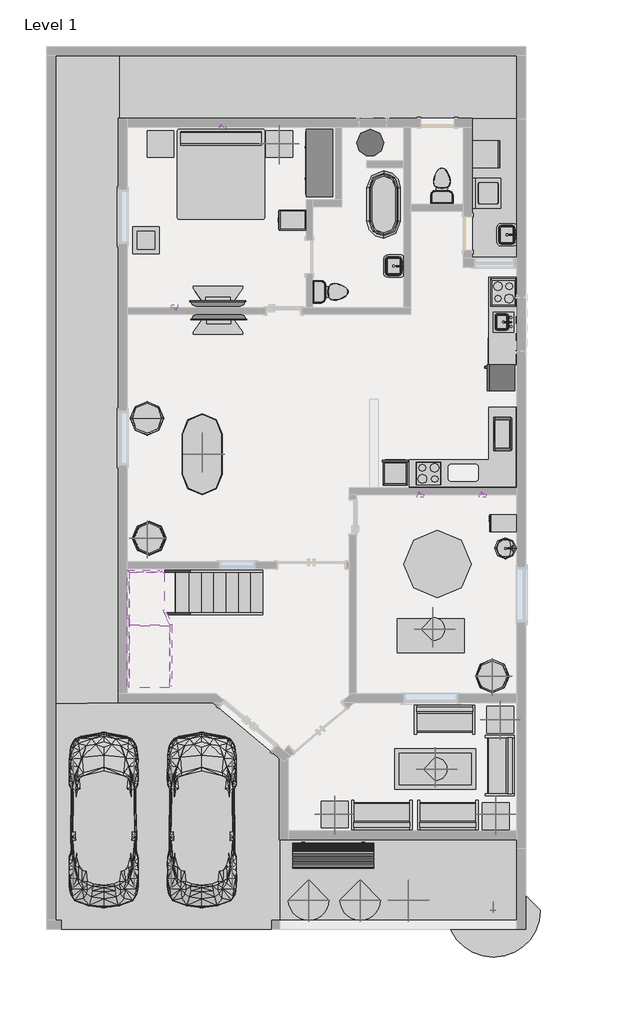
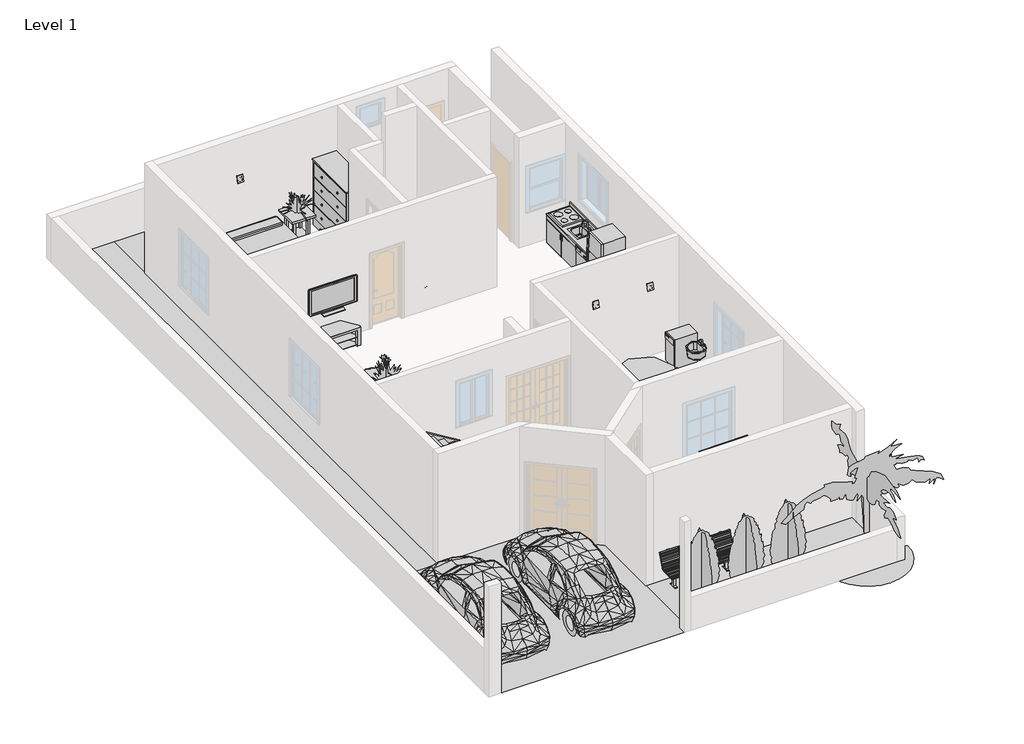
# One storey, part 2 of 2: 26 furniture elements, 21 proxies, 14 geographic elements, 8 flow terminals, 7 members, 2 stair flights, 1 slab.
"""IFC4 building model written with IfcOpenShell, lengths in millimetres."""

from ifc_helpers import new_model, si_unit, frame, origin, place, context, project, spatial, polyline, outline, extrude, faceted_brep, triangles, transform, mapped, element, save
from components import proxy_db4bb64d, proxy_a6faaae8, proxy_45b28599, kitchenette_medium_kitchenette_medium_844211aa, proxy_8a8d5ab2, proxy_8b8c2dc4, rpc_beetle_rpc_beetle_3ce7ba48, rpc_picture_frame_rpc_picture_frame_c25e3fe9, proxy_c523a7b7, proxy_718fa39f, flow_terminal_871c2e40, flow_terminal_d49f872f, flow_terminal_62a433f7, toilet_domestic_3d_toilet_domestic_3d_f7549cf7, toilet_domestic_3d_toilet_domestic_3d_183bbd19, flow_terminal_b374fae2, water_heater_water_heater_e0cc5f81, furniture_3a47f844, furniture_1fc5af50, furniture_c6510c7c, furniture_eb5480b5, furniture_d0678273, furniture_22419f35, furniture_fdf74506, tv_stand_tv_stand_6ce107e5, furniture_b5c51a22, furniture_cd93a443, furniture_37c8c8f5, furniture_2c34a4f9, furniture_bbcc68ce, furniture_5bc9ed15, furniture_ebfaaaa6, geographic_element_235d1464, rpc_plant_tropical_55f6ff97, rpc_plant_tropical_agave_1_5_93a2a214, rpc_plant_tropical_dagger_2_80c14bd7, rpc_tree_conifer_chinese_juniper_7_1b9786cd, rpc_tree_tropical_australian_tree_furn_6_f1eb339c, non_monolithic_landing_fae4903c, stair_flight_6609341a, stair_flight_531346ed

model = new_model("IFC4")

# Units and contexts
model_context = context("Model", 3, world=origin())
ifc_project = project(units=[si_unit("LENGTHUNIT", "METRE", prefix="MILLI")], contexts=[model_context])

# Site, building, storey
site = spatial("IfcSite", under=ifc_project)
building = spatial("IfcBuilding", under=site)
storey = spatial("IfcBuildingStorey", under=building, Name="Level 1", Elevation=0.0)

# Proxies
placement = place(None, origin())
element("IfcBuildingElementProxy", 1, Name="Building Element Proxy", at=placement, inside=storey, context=model_context, shape_type="Tessellation", body=[
    triangles([(-7203.0899826, -1251.0682583, 0.0), (-7195.9601852, -3079.8684036, 0.0), (-1811.1602337, -3079.8684036, 0.0), (-1811.1602337, -1251.0682583, 0.0)], [[1, 2, 4], [3, 4, 2]], closed=False),
])
element("IfcBuildingElementProxy", 2, Name="Building Element Proxy", at=placement, inside=storey, context=model_context, shape_type="Tessellation", body=[
    triangles([(-7203.0899826, -1251.0682583, 0.0), (-12275.9599915, -1235.8155556, 0.0), (-12275.9599915, -3079.8684036, 0.0), (-7373.760379, -3079.8684036, 0.0), (-7373.760379, -3283.0682098, 0.0), (-12148.9607666, -3283.0682098, 0.0), (-7203.0899826, 588.2438181, 0.0), (-8706.1017288, 1847.7316933, 0.0), (-10853.5607666, 1847.7316933, 0.0), (-12275.9599915, 1824.0178791, 0.0), (-7204.4183899, -2110.1262875, 0.0), (-7195.9601852, -3079.8684036, 0.0)], [[3, 6, 2], [8, 2, 1], [6, 4, 11], [2, 9, 10], [9, 2, 8], [2, 6, 11], [4, 5, 12], [5, 4, 6], [4, 12, 11], [7, 8, 1], [1, 11, 12], [7, 1, 12], [2, 11, 1]], closed=False),
])
element("IfcBuildingElementProxy", 3, Name="Building Element Proxy", at=placement, inside=storey, context=model_context, shape_type="Tessellation", body=[
    triangles([(-12275.9599915, 1818.2510799, 0.0), (-10853.5607666, 1847.7316933, 0.0), (-10853.5607666, 15106.5314026, 0.0), (-10835.0514313, 16528.9317902, 0.0), (-12275.9599915, 16528.9317902, 0.0)], [[5, 1, 3], [3, 2, 4], [2, 3, 1], [3, 4, 5]], closed=False),
])
element("IfcBuildingElementProxy", 4, Name="Building Element Proxy", at=placement, inside=storey, context=model_context, shape_type="Tessellation", body=[
    triangles([(-10853.5607666, 15106.5314026, 0.0), (-10833.5468719, 16528.9317902, 0.0), (-1811.1602337, 16528.9317902, 0.0), (-1811.1602337, 15106.5314026, 0.0)], [[2, 1, 4], [4, 3, 2]], closed=False),
])
element("IfcBuildingElementProxy", 5, Name="Building Element Proxy", at=placement, inside=storey, context=model_context, shape_type="Tessellation", body=[
    triangles([(-2827.1602821, 12160.1321777, 0.0), (-1811.1602337, 12160.1321777, 0.0), (-1811.1602337, 15081.1317902, 0.0), (-1811.1602337, 15106.5314026, 0.0), (-2827.1602821, 15106.5314026, 0.0), (-2827.1602821, 11956.9317902, 0.0), (-1927.5673725, 11950.5821777, 0.0), (-1931.5440193, 11943.2954132, 0.0), (-2807.9911034, 11944.0976898, 0.0), (-1804.8101852, 11950.5821777, 0.0)], [[9, 8, 1], [3, 1, 2], [1, 6, 9], [3, 5, 1], [1, 8, 7], [7, 10, 2], [10, 7, 8], [10, 3, 2], [1, 7, 2], [4, 5, 3]], closed=False),
])
proxy_shape = proxy_db4bb64d(model_context)
element("IfcBuildingElementProxy", 6, Name="15\" x 24\" x 34 1/2\"", ObjectType="15\" x 24\" x 34 1/2\"", at=placement, inside=storey, context=model_context, shape_type="MappedRepresentation", body=[
    mapped(proxy_shape, transform((-2382.4098076, 6192.4491673, 0.0), x_axis=(0.0, -1.0000000000000004, 0.0), y_axis=(1.0000000000000004, 0.0, 0.0), z_axis=(0.0, 0.0, 1.0))),
])
proxy_2_shape = proxy_a6faaae8(model_context)
element("IfcBuildingElementProxy", 7, Name="Cook Top-4 Unit2 : 22\" x 20\"", ObjectType="Cook Top-4 Unit2 : 22\" x 20\"", at=placement, inside=storey, context=model_context, shape_type="MappedRepresentation", body=[
    mapped(proxy_2_shape, transform((-2115.9602428, 11156.8316988, 0.0), x_axis=(0.0, -1.0000000000000004, 0.0), y_axis=(1.0000000000000004, 0.0, 0.0), z_axis=(0.0, 0.0, 1.0))),
])
element("IfcBuildingElementProxy", 8, Name="Cook Top-4 Unit2 : 22\" x 20\"", ObjectType="Cook Top-4 Unit2 : 22\" x 20\"", at=placement, inside=storey, context=model_context, shape_type="MappedRepresentation", body=[
    mapped(proxy_2_shape, transform((-3817.7602428, 7054.7316988, 0.0), x_axis=(1.0, 0.0, 0.0), y_axis=(0.0, 1.0, 0.0), z_axis=(0.0, 0.0, 1.0))),
])
proxy_3_shape = proxy_45b28599(model_context)
element("IfcBuildingElementProxy", 9, Name="Dishwasher : 24\" x 24\" x 34\"", ObjectType="Dishwasher : 24\" x 24\" x 34\"", at=placement, inside=storey, context=model_context, shape_type="MappedRepresentation", body=[
    mapped(proxy_3_shape, transform((-2407.8098076, 10205.6491673, 0.0), x_axis=(0.0, -1.0000000000000004, 0.0), y_axis=(1.0000000000000004, 0.0, 0.0), z_axis=(0.0, 0.0, 1.0))),
])
element("IfcBuildingElementProxy", 10, Name="Dishwasher : 24\" x 24\" x 34\"", ObjectType="Dishwasher : 24\" x 24\" x 34\"", at=placement, inside=storey, context=model_context, shape_type="MappedRepresentation", body=[
    mapped(proxy_3_shape, transform((-2255.910678, 13911.4142303, 0.0), x_axis=(0.0, 1.0, 0.0), y_axis=(-1.0, 0.0, 0.0), z_axis=(0.0, 0.0, 1.0))),
])
kitchenette_medium_kitchenette_medium_shape = kitchenette_medium_kitchenette_medium_844211aa(model_context)
element("IfcBuildingElementProxy", 11, Name="Kitchenette - Medium : Kitchenette - Medium", ObjectType="Kitchenette - Medium : Kitchenette - Medium", at=placement, inside=storey, context=model_context, shape_type="MappedRepresentation", body=[
    mapped(kitchenette_medium_kitchenette_medium_shape, transform((-1811.1602428, 10832.6694037, 0.0), x_axis=(0.0, -1.0000000000000004, 0.0), y_axis=(1.0000000000000004, 0.0, 0.0), z_axis=(0.0, 0.0, 1.0))),
])
proxy_4_shape = proxy_8a8d5ab2(model_context)
element("IfcBuildingElementProxy", 12, Name="Microwave : 30\" x 16\" x 18\"", ObjectType="Microwave : 30\" x 16\" x 18\"", at=placement, inside=storey, context=model_context, shape_type="MappedRepresentation", body=[
    mapped(proxy_4_shape, transform((-1779.2383078, 8444.0245761, 0.0), x_axis=(0.0, -1.0000000000000004, 0.0), y_axis=(1.0000000000000004, 0.0, 0.0), z_axis=(0.0, 0.0, 1.0))),
])
proxy_5_shape = proxy_8b8c2dc4(model_context)
element("IfcBuildingElementProxy", 13, Name="Oven Double-Built-in : 21 1/2\" x 39 1/4\" x 21\"", ObjectType="Oven Double-Built-in : 21 1/2\" x 39 1/4\" x 21\"", at=placement, inside=storey, context=model_context, shape_type="MappedRepresentation", body=[
    mapped(proxy_5_shape, transform((-4605.8937409, 7195.7975577, 0.0), x_axis=(-1.0, 0.0, 0.0), y_axis=(0.0, -1.0, 0.0), z_axis=(0.0, 0.0, 1.0))),
])
rpc_beetle_rpc_beetle_shape = rpc_beetle_rpc_beetle_3ce7ba48(model_context)
element("IfcBuildingElementProxy", 14, Name="RPC Beetle : RPC Beetle", ObjectType="RPC Beetle : RPC Beetle", at=placement, inside=storey, context=model_context, shape_type="MappedRepresentation", body=[
    mapped(rpc_beetle_rpc_beetle_shape, transform((-11183.7602428, -2038.4683012, 0.0), x_axis=(1.0, 0.0, 0.0), y_axis=(0.0, 1.0, 0.0), z_axis=(0.0, 0.0, 1.0))),
])
element("IfcBuildingElementProxy", 15, Name="RPC Beetle : RPC Beetle", ObjectType="RPC Beetle : RPC Beetle", at=placement, inside=storey, context=model_context, shape_type="MappedRepresentation", body=[
    mapped(rpc_beetle_rpc_beetle_shape, transform((-8955.6900205, -2038.4683012, 0.0), x_axis=(1.0, 0.0, 0.0), y_axis=(0.0, 1.0, 0.0), z_axis=(0.0, 0.0, 1.0))),
])
rpc_picture_frame_rpc_picture_frame_shape = rpc_picture_frame_rpc_picture_frame_c25e3fe9(model_context)
element("IfcBuildingElementProxy", 16, Name="RPC Picture Frame : RPC Picture Frame", ObjectType="RPC Picture Frame : RPC Picture Frame", at=placement, inside=storey, context=model_context, shape_type="MappedRepresentation", body=[
    mapped(rpc_picture_frame_rpc_picture_frame_shape, transform((-9578.1095933, 10813.9316988, 1828.8), x_axis=(-1.0000000000000004, 0.0, 0.0), y_axis=(0.0, -1.0000000000000004, 0.0), z_axis=(0.0, 0.0, 1.0))),
])
element("IfcBuildingElementProxy", 17, Name="RPC Picture Frame : RPC Picture Frame", ObjectType="RPC Picture Frame : RPC Picture Frame", at=placement, inside=storey, context=model_context, shape_type="MappedRepresentation", body=[
    mapped(rpc_picture_frame_rpc_picture_frame_shape, transform((-8489.5300722, 14903.3316988, 1828.8), x_axis=(1.0, 0.0, 0.0), y_axis=(0.0, 1.0, 0.0), z_axis=(0.0, 0.0, 1.0))),
])
element("IfcBuildingElementProxy", 18, Name="RPC Picture Frame : RPC Picture Frame", ObjectType="RPC Picture Frame : RPC Picture Frame", at=placement, inside=storey, context=model_context, shape_type="MappedRepresentation", body=[
    mapped(rpc_picture_frame_rpc_picture_frame_shape, transform((-4002.0994377, 6572.1316988, 1828.8), x_axis=(1.0, 0.0, 0.0), y_axis=(0.0, 1.0, 0.0), z_axis=(0.0, 0.0, 1.0))),
])
element("IfcBuildingElementProxy", 19, Name="RPC Picture Frame : RPC Picture Frame", ObjectType="RPC Picture Frame : RPC Picture Frame", at=placement, inside=storey, context=model_context, shape_type="MappedRepresentation", body=[
    mapped(rpc_picture_frame_rpc_picture_frame_shape, transform((-2586.2560744, 6572.1316988, 1828.8), x_axis=(1.0, 0.0, 0.0), y_axis=(0.0, 1.0, 0.0), z_axis=(0.0, 0.0, 1.0))),
])
proxy_6_shape = proxy_c523a7b7(model_context)
element("IfcBuildingElementProxy", 20, Name="Refrigerator : 24\" x 25\" LH", ObjectType="Refrigerator : 24\" x 25\" LH", at=placement, inside=storey, context=model_context, shape_type="MappedRepresentation", body=[
    mapped(proxy_6_shape, transform((-2161.6092143, 9220.0816988, 0.0), x_axis=(0.0, -1.0000000000000004, 0.0), y_axis=(1.0000000000000004, 0.0, 0.0), z_axis=(0.0, 0.0, 1.0))),
])
proxy_7_shape = proxy_718fa39f(model_context)
element("IfcBuildingElementProxy", 21, Name="Washer : 27\" x 25\" x 35\"", ObjectType="Washer : 27\" x 25\" x 35\"", at=placement, inside=storey, context=model_context, shape_type="MappedRepresentation", body=[
    mapped(proxy_7_shape, transform((-2216.2427743, 12985.3812636, 0.0), x_axis=(0.0, 1.0000000000000009, 0.0), y_axis=(-1.0000000000000009, 0.0, 0.0), z_axis=(0.0, 0.0, 1.0))),
])

# Flow terminals
flow_terminal_shape = flow_terminal_871c2e40(model_context)
element("IfcFlowTerminal", 22, ObjectType="Sink Kitchen-Island : 18\" x 18\"", at=placement, inside=storey, context=model_context, shape_type="MappedRepresentation", body=[
    mapped(flow_terminal_shape, transform((-2118.3056439, 10499.4209394, -14.4), x_axis=(0.0, -1.0000000000000004, 0.0), y_axis=(1.0000000000000004, 0.0, 0.0), z_axis=(0.0, 0.0, 1.0))),
])
flow_terminal_2_shape = flow_terminal_d49f872f(model_context)
element("IfcFlowTerminal", 23, ObjectType="Sink Vanity-Round : 19\" x 19\"", at=placement, inside=storey, context=model_context, shape_type="MappedRepresentation", body=[
    mapped(flow_terminal_2_shape, transform((-2157.9067046, 5449.5834394, 0.0), x_axis=(0.0, -1.0000000000000004, 0.0), y_axis=(1.0000000000000004, 0.0, 0.0), z_axis=(0.0, 0.0, 1.0))),
])
flow_terminal_3_shape = flow_terminal_62a433f7(model_context)
element("IfcFlowTerminal", 24, ObjectType="Sink Vanity-Square : 20\" x 18\"", at=placement, inside=storey, context=model_context, shape_type="MappedRepresentation", body=[
    mapped(flow_terminal_3_shape, transform((-4556.7056439, 11769.4209394, 0.0), x_axis=(0.0, -1.0, 0.0), y_axis=(1.0, 0.0, 0.0), z_axis=(0.0, 0.0, 1.0))),
])
element("IfcFlowTerminal", 25, ObjectType="Sink Vanity-Square : 20\" x 18\"", at=placement, inside=storey, context=model_context, shape_type="MappedRepresentation", body=[
    mapped(flow_terminal_3_shape, transform((-1991.3056439, 12480.6209394, 0.0), x_axis=(0.0, -1.0000000000000007, 0.0), y_axis=(1.0000000000000007, 0.0, 0.0), z_axis=(0.0, 0.0, 1.0))),
])
toilet_domestic_3d_toilet_domestic_3d_shape = toilet_domestic_3d_toilet_domestic_3d_f7549cf7(model_context)
toilet_domestic_3d_toilet_domestic_3d_2_shape = toilet_domestic_3d_toilet_domestic_3d_183bbd19(model_context)
element("IfcFlowTerminal", 26, ObjectType="Toilet-Domestic-3D : Toilet-Domestic-3D", at=placement, inside=storey, context=model_context, shape_type="MappedRepresentation", body=[
    mapped(toilet_domestic_3d_toilet_domestic_3d_shape, transform((-5946.3939931, 11169.5316988, 0.0), x_axis=(0.0, 0.9999999999999999, 0.0), y_axis=(-0.9999999999999999, 0.0, 0.0), z_axis=(0.0, 0.0, 1.0))),
    mapped(toilet_domestic_3d_toilet_domestic_3d_2_shape, transform((-5946.3939931, 11169.5316988, 0.0), x_axis=(0.0, 0.9999999999999999, 0.0), y_axis=(-0.9999999999999999, 0.0, 0.0), z_axis=(0.0, 0.0, 1.0))),
])
element("IfcFlowTerminal", 27, ObjectType="Toilet-Domestic-3D : Toilet-Domestic-3D", at=placement, inside=storey, context=model_context, shape_type="MappedRepresentation", body=[
    mapped(toilet_domestic_3d_toilet_domestic_3d_shape, transform((-3512.9602428, 13670.8277261, 0.0), x_axis=(-1.0000000000000004, 0.0, 0.0), y_axis=(0.0, -1.0000000000000004, 0.0), z_axis=(0.0, 0.0, 1.0))),
    mapped(toilet_domestic_3d_toilet_domestic_3d_2_shape, transform((-3512.9602428, 13670.8277261, 0.0), x_axis=(-1.0000000000000004, 0.0, 0.0), y_axis=(0.0, -1.0000000000000004, 0.0), z_axis=(0.0, 0.0, 1.0))),
])
flow_terminal_4_shape = flow_terminal_b374fae2(model_context)
element("IfcFlowTerminal", 28, ObjectType="Tub-Free Standing-3D : 30\" x 60\"", at=placement, inside=storey, context=model_context, shape_type="MappedRepresentation", body=[
    mapped(flow_terminal_4_shape, transform((-4833.7602428, 13150.7316988, 0.0), x_axis=(1.0000000000000007, 0.0, 0.0), y_axis=(0.0, 1.0000000000000007, 0.0), z_axis=(0.0, 0.0, 1.0))),
])
water_heater_water_heater_shape = water_heater_water_heater_e0cc5f81(model_context)
element("IfcFlowTerminal", 29, ObjectType="Water Heater : Water Heater", at=placement, inside=storey, context=model_context, shape_type="MappedRepresentation", body=[
    mapped(water_heater_water_heater_shape, transform((-5138.4319947, 14547.7316988, 0.0), x_axis=(1.0, 0.0, 0.0), y_axis=(0.0, 1.0, 0.0), z_axis=(0.0, 0.0, 1.0))),
])

# Furniture
furniture_shape = furniture_3a47f844(model_context)
element("IfcFurniture", 30, ObjectType="Base Cabinet-2 Bin : 18\"", at=placement, inside=storey, context=model_context, shape_type="MappedRepresentation", body=[
    mapped(furniture_shape, transform((-6593.4900205, 12776.3939939, 0.0), x_axis=(0.0, 1.0000000000000002, 0.0), y_axis=(-1.0000000000000002, 0.0, 0.0), z_axis=(0.0, 0.0, 1.0))),
])
furniture_2_shape = furniture_1fc5af50(model_context)
element("IfcFurniture", 31, ObjectType="Bed-Standard.0001 : King 78\" x 80\"", at=placement, inside=storey, context=model_context, shape_type="MappedRepresentation", body=[
    mapped(furniture_2_shape, transform((-8795.3785451, 13882.1267808, 0.0), x_axis=(1.0, 0.0, 0.0), y_axis=(0.0, 1.0, 0.0), z_axis=(0.0, 0.0, 1.0))),
])
furniture_3_shape = furniture_c6510c7c(model_context)
element("IfcFurniture", 32, ObjectType="Counter Top w Sink Hole : 24\" Depth", at=placement, inside=storey, context=model_context, shape_type="MappedRepresentation", body=[
    mapped(furniture_3_shape, transform((-1811.1602428, 10299.2694037, -14.4), x_axis=(0.0, -1.0000000000000004, 0.0), y_axis=(1.0000000000000004, 0.0, 0.0), z_axis=(0.0, 0.0, 1.0))),
])
furniture_4_shape = furniture_eb5480b5(model_context)
element("IfcFurniture", 33, ObjectType="Counter Top-L Shaped w Sink Hole : 24\" Depth", at=placement, inside=storey, context=model_context, shape_type="MappedRepresentation", body=[
    mapped(furniture_4_shape, transform((-3011.6225379, 6724.5316988, 0.0), x_axis=(-1.0000000000000002, 0.0, 0.0), y_axis=(0.0, -1.0000000000000002, 0.0), z_axis=(0.0, 0.0, 1.0))),
])
furniture_5_shape = furniture_d0678273(model_context)
element("IfcFurniture", 34, ObjectType="Dresser : 48\" x 72\" x 24\"", at=placement, inside=storey, context=model_context, shape_type="MappedRepresentation", body=[
    mapped(furniture_5_shape, transform((-5925.5270664, 13821.338439, 0.0), x_axis=(0.0, -1.0000000000000004, 0.0), y_axis=(1.0000000000000004, 0.0, 0.0), z_axis=(0.0, 0.0, 1.0))),
])
furniture_6_shape = furniture_22419f35(model_context)
element("IfcFurniture", 35, ObjectType="Sofa : 54\"", at=placement, inside=storey, context=model_context, shape_type="MappedRepresentation", body=[
    mapped(furniture_6_shape, transform((-3523.4893054, 1320.5776004, 0.0), x_axis=(1.0, 0.0, 0.0), y_axis=(0.0, 1.0, 0.0), z_axis=(0.0, 0.0, 1.0))),
])
element("IfcFurniture", 36, ObjectType="Sofa : 54\"", at=placement, inside=storey, context=model_context, shape_type="MappedRepresentation", body=[
    mapped(furniture_6_shape, transform((-2344.6643411, 495.7021906, 0.0), x_axis=(0.0, -1.0000000000000004, 0.0), y_axis=(1.0000000000000004, 0.0, 0.0), z_axis=(0.0, 0.0, 1.0))),
])
element("IfcFurniture", 37, ObjectType="Sofa : 54\"", at=placement, inside=storey, context=model_context, shape_type="MappedRepresentation", body=[
    mapped(furniture_6_shape, transform((-3306.5483218, -546.1142028, 0.0), x_axis=(-1.0000000000000002, 0.0, 0.0), y_axis=(0.0, -1.0000000000000002, 0.0), z_axis=(0.0, 0.0, 1.0))),
])
element("IfcFurniture", 38, ObjectType="Sofa : 54\"", at=placement, inside=storey, context=model_context, shape_type="MappedRepresentation", body=[
    mapped(furniture_6_shape, transform((-4805.1483218, -546.1142028, 0.0), x_axis=(-1.0, 0.0, 0.0), y_axis=(0.0, -1.0, 0.0), z_axis=(0.0, 0.0, 1.0))),
])
furniture_7_shape = furniture_fdf74506(model_context)
element("IfcFurniture", 39, ObjectType="TV - Flat Screen : 50\"", at=placement, inside=storey, context=model_context, shape_type="MappedRepresentation", body=[
    mapped(furniture_7_shape, transform((-8596.9047569, 10897.8703224, 914.4), x_axis=(-1.0, 0.0, 0.0), y_axis=(0.0, -1.0, 0.0), z_axis=(0.0, 0.0, 1.0))),
])
element("IfcFurniture", 40, ObjectType="TV - Flat Screen : 50\"", at=placement, inside=storey, context=model_context, shape_type="MappedRepresentation", body=[
    mapped(furniture_7_shape, transform((-8570.7455063, 10602.9930751, 914.4), x_axis=(1.0, 0.0, 0.0), y_axis=(0.0, 1.0, 0.0), z_axis=(0.0, 0.0, 1.0))),
])
tv_stand_tv_stand_shape = tv_stand_tv_stand_6ce107e5(model_context)
element("IfcFurniture", 41, ObjectType="TV Stand : TV Stand", at=placement, inside=storey, context=model_context, shape_type="MappedRepresentation", body=[
    mapped(tv_stand_tv_stand_shape, transform((-8467.7722407, 10839.3316988, 0.0), x_axis=(-1.0, 0.0, 0.0), y_axis=(0.0, -1.0, 0.0), z_axis=(0.0, 0.0, 1.0))),
])
element("IfcFurniture", 42, ObjectType="TV Stand : TV Stand", at=placement, inside=storey, context=model_context, shape_type="MappedRepresentation", body=[
    mapped(tv_stand_tv_stand_shape, transform((-8718.1482448, 10661.5316988, 0.0), x_axis=(1.0, 0.0, 0.0), y_axis=(0.0, 1.0, 0.0), z_axis=(0.0, 0.0, 1.0))),
])
furniture_8_shape = furniture_b5c51a22(model_context)
element("IfcFurniture", 43, ObjectType="Table-Coffee : 24\" x 24\" x 24\"", at=placement, inside=storey, context=model_context, shape_type="MappedRepresentation", body=[
    mapped(furniture_8_shape, transform((-10242.5814222, 12242.720621, 0.0), x_axis=(1.0, 0.0, 0.0), y_axis=(0.0, 1.0, 0.0), z_axis=(0.0, 0.0, 1.0))),
])
furniture_9_shape = furniture_cd93a443(model_context)
element("IfcFurniture", 44, ObjectType="Table-Coffee : 36\" x 72\" x 18\"", at=placement, inside=storey, context=model_context, shape_type="MappedRepresentation", body=[
    mapped(furniture_9_shape, transform((-3683.6260094, 253.920621, 0.0), x_axis=(1.0, 0.0, 0.0), y_axis=(0.0, 1.0, 0.0), z_axis=(0.0, 0.0, 1.0))),
])
furniture_10_shape = furniture_37c8c8f5(model_context)
element("IfcFurniture", 45, ObjectType="Table-Dining : 30\" x 84\" x 22\"", at=placement, inside=storey, context=model_context, shape_type="MappedRepresentation", body=[
    mapped(furniture_10_shape, transform((-3785.2260094, 3276.520621, 0.0), x_axis=(1.0, 0.0, 0.0), y_axis=(0.0, 1.0, 0.0), z_axis=(0.0, 0.0, 1.0))),
])
furniture_11_shape = furniture_2c34a4f9(model_context)
element("IfcFurniture", 46, ObjectType="Table-Dining Oval : 36\" x 72\"", at=placement, inside=storey, context=model_context, shape_type="MappedRepresentation", body=[
    mapped(furniture_11_shape, transform((-9306.6586034, 7888.3513709, 0.0), x_axis=(0.0, 1.0, 0.0), y_axis=(-1.0, 0.0, 0.0), z_axis=(0.0, 0.0, 1.0))),
])
furniture_12_shape = furniture_bbcc68ce(model_context)
element("IfcFurniture", 47, ObjectType="Table-Dining Round w Chairs : 60\" Diameter", at=placement, inside=storey, context=model_context, shape_type="MappedRepresentation", body=[
    mapped(furniture_12_shape, transform((-3718.24221, 5182.2103873, 0.0), x_axis=(1.0, 0.0, 0.0), y_axis=(0.0, 1.0, 0.0), z_axis=(0.0, 0.0, 1.0))),
])
furniture_13_shape = furniture_5bc9ed15(model_context)
element("IfcFurniture", 48, ObjectType="Table-Night Stand : 24\" x 24\" x 30\"", at=placement, inside=storey, context=model_context, shape_type="MappedRepresentation", body=[
    mapped(furniture_13_shape, transform((-10204.0236508, 14217.5316988, 0.0), x_axis=(1.0, 0.0, 0.0), y_axis=(0.0, 1.0, 0.0), z_axis=(0.0, 0.0, 1.0))),
])
element("IfcFurniture", 49, ObjectType="Table-Night Stand : 24\" x 24\" x 30\"", at=placement, inside=storey, context=model_context, shape_type="MappedRepresentation", body=[
    mapped(furniture_13_shape, transform((-7511.6236508, 14217.5316988, 0.0), x_axis=(1.0, 0.0, 0.0), y_axis=(0.0, 1.0, 0.0), z_axis=(0.0, 0.0, 1.0))),
])
element("IfcFurniture", 50, ObjectType="Table-Night Stand : 24\" x 24\" x 30\"", at=placement, inside=storey, context=model_context, shape_type="MappedRepresentation", body=[
    mapped(furniture_13_shape, transform((-1985.2266125, -412.8683012, 0.0), x_axis=(-1.0000000000000004, 0.0, 0.0), y_axis=(0.0, -1.0000000000000004, 0.0), z_axis=(0.0, 0.0, 1.0))),
])
element("IfcFurniture", 51, ObjectType="Table-Night Stand : 24\" x 24\" x 30\"", at=placement, inside=storey, context=model_context, shape_type="MappedRepresentation", body=[
    mapped(furniture_13_shape, transform((-2500.6938731, 1161.9316988, 0.0), x_axis=(1.0, 0.0, 0.0), y_axis=(0.0, 1.0, 0.0), z_axis=(0.0, 0.0, 1.0))),
])
element("IfcFurniture", 52, ObjectType="Table-Night Stand : 24\" x 24\" x 30\"", at=placement, inside=storey, context=model_context, shape_type="MappedRepresentation", body=[
    mapped(furniture_13_shape, transform((-6250.8524439, -985.8982957, 0.0), x_axis=(1.0, 0.0, 0.0), y_axis=(0.0, 1.0, 0.0), z_axis=(0.0, 0.0, 1.0))),
])
furniture_14_shape = furniture_ebfaaaa6(model_context)
element("IfcFurniture", 53, ObjectType="Table-Round : 36\" Diameter", at=placement, inside=storey, context=model_context, shape_type="MappedRepresentation", body=[
    mapped(furniture_14_shape, transform((-2369.9602428, 2457.3316988, 0.0), x_axis=(1.0, 0.0, 0.0), y_axis=(0.0, 1.0, 0.0), z_axis=(0.0, 0.0, 1.0))),
])
element("IfcFurniture", 54, ObjectType="Table-Round : 36\" Diameter", at=placement, inside=storey, context=model_context, shape_type="MappedRepresentation", body=[
    mapped(furniture_14_shape, transform((-10149.4900205, 5581.5316988, 0.0), x_axis=(1.0, 0.0, 0.0), y_axis=(0.0, 1.0, 0.0), z_axis=(0.0, 0.0, 1.0))),
])
element("IfcFurniture", 55, ObjectType="Table-Round : 36\" Diameter", at=placement, inside=storey, context=model_context, shape_type="MappedRepresentation", body=[
    mapped(furniture_14_shape, transform((-10200.2900205, 8299.3316988, 0.0), x_axis=(1.0, 0.0, 0.0), y_axis=(0.0, 1.0, 0.0), z_axis=(0.0, 0.0, 1.0))),
])

# Geographic elements
geographic_element_shape = geographic_element_235d1464(model_context)
element("IfcGeographicElement", 56, ObjectType="Park Bench : 72\"", at=placement, inside=storey, context=model_context, shape_type="MappedRepresentation", body=[
    mapped(geographic_element_shape, transform((-5976.7602428, -1581.2683012, 0.0), x_axis=(1.0, 0.0, 0.0), y_axis=(0.0, 1.0, 0.0), z_axis=(0.0, 0.0, 1.0))),
])
rpc_plant_tropical_shape = rpc_plant_tropical_55f6ff97(model_context)
element("IfcGeographicElement", 57, ObjectType="RPC Plant - Tropical", at=placement, inside=storey, context=model_context, shape_type="MappedRepresentation", body=[
    mapped(rpc_plant_tropical_shape, transform((-3665.3602428, 349.1316988, 762.0), x_axis=(0.0, 1.0, 0.0), y_axis=(-1.0, 0.0, 0.0), z_axis=(0.0, 0.0, 1.0))),
])
element("IfcGeographicElement", 58, ObjectType="RPC Plant - Tropical", at=placement, inside=storey, context=model_context, shape_type="MappedRepresentation", body=[
    mapped(rpc_plant_tropical_shape, transform((-3716.1602428, 3524.1316988, 762.0), x_axis=(0.0, 1.0000000000000002, 0.0), y_axis=(-1.0000000000000002, 0.0, 0.0), z_axis=(0.0, 0.0, 1.0))),
])
element("IfcGeographicElement", 59, ObjectType="RPC Plant - Tropical", at=placement, inside=storey, context=model_context, shape_type="MappedRepresentation", body=[
    mapped(rpc_plant_tropical_shape, transform((-8948.5602428, 7486.5316988, 762.0), x_axis=(0.0, 1.0000000000000002, 0.0), y_axis=(-1.0000000000000002, 0.0, 0.0), z_axis=(0.0, 0.0, 1.0))),
])
rpc_plant_tropical_agave_1_5_shape = rpc_plant_tropical_agave_1_5_93a2a214(model_context)
element("IfcGeographicElement", 60, ObjectType="RPC Plant - Tropical : Agave - 1.5'", at=placement, inside=storey, context=model_context, shape_type="MappedRepresentation", body=[
    mapped(rpc_plant_tropical_agave_1_5_shape, transform((-5942.3188136, -681.0982957, 762.0), x_axis=(1.0, 0.0, 0.0), y_axis=(0.0, 1.0, 0.0), z_axis=(0.0, 0.0, 1.0))),
])
element("IfcGeographicElement", 61, ObjectType="RPC Plant - Tropical : Agave - 1.5'", at=placement, inside=storey, context=model_context, shape_type="MappedRepresentation", body=[
    mapped(rpc_plant_tropical_agave_1_5_shape, transform((-2293.7602428, -681.0982957, 762.0), x_axis=(1.0, 0.0, 0.0), y_axis=(0.0, 1.0, 0.0), z_axis=(0.0, 0.0, 1.0))),
])
element("IfcGeographicElement", 62, ObjectType="RPC Plant - Tropical : Agave - 1.5'", at=placement, inside=storey, context=model_context, shape_type="MappedRepresentation", body=[
    mapped(rpc_plant_tropical_agave_1_5_shape, transform((-2192.1602428, 1466.7316988, 0.0), x_axis=(1.0, 0.0, 0.0), y_axis=(0.0, 1.0, 0.0), z_axis=(0.0, 0.0, 1.0))),
])
element("IfcGeographicElement", 63, ObjectType="RPC Plant - Tropical : Agave - 1.5'", at=placement, inside=storey, context=model_context, shape_type="MappedRepresentation", body=[
    mapped(rpc_plant_tropical_agave_1_5_shape, transform((-7203.0900205, 14522.3316988, 762.0), x_axis=(1.0, 0.0, 0.0), y_axis=(0.0, 1.0, 0.0), z_axis=(0.0, 0.0, 1.0))),
])
rpc_plant_tropical_dagger_2_shape = rpc_plant_tropical_dagger_2_80c14bd7(model_context)
element("IfcGeographicElement", 64, ObjectType="RPC Plant - Tropical : Dagger - 2'", at=placement, inside=storey, context=model_context, shape_type="MappedRepresentation", body=[
    mapped(rpc_plant_tropical_dagger_2_shape, transform((-2369.9602428, 2457.3316988, 762.0), x_axis=(1.0, 0.0, 0.0), y_axis=(0.0, 1.0, 0.0), z_axis=(0.0, 0.0, 1.0))),
])
element("IfcGeographicElement", 65, ObjectType="RPC Plant - Tropical : Dagger - 2'", at=placement, inside=storey, context=model_context, shape_type="MappedRepresentation", body=[
    mapped(rpc_plant_tropical_dagger_2_shape, transform((-10200.2900205, 5581.5316988, 762.0), x_axis=(1.0, 0.0, 0.0), y_axis=(0.0, 1.0, 0.0), z_axis=(0.0, 0.0, 1.0))),
])
rpc_tree_conifer_chinese_juniper_7_shape = rpc_tree_conifer_chinese_juniper_7_1b9786cd(model_context)
element("IfcGeographicElement", 66, ObjectType="RPC Tree - Conifer : Chinese Juniper - 7'", at=placement, inside=storey, context=model_context, shape_type="MappedRepresentation", body=[
    mapped(rpc_tree_conifer_chinese_juniper_7_shape, transform((-6535.7569139, -2622.6683012, 0.0), x_axis=(1.0, 0.0, 0.0), y_axis=(0.0, 1.0, 0.0), z_axis=(0.0, 0.0, 1.0))),
])
element("IfcGeographicElement", 67, ObjectType="RPC Tree - Conifer : Chinese Juniper - 7'", at=placement, inside=storey, context=model_context, shape_type="MappedRepresentation", body=[
    mapped(rpc_tree_conifer_chinese_juniper_7_shape, transform((-5367.3569139, -2622.6683012, 0.0), x_axis=(1.0, 0.0, 0.0), y_axis=(0.0, 1.0, 0.0), z_axis=(0.0, 0.0, 1.0))),
])
element("IfcGeographicElement", 68, ObjectType="RPC Tree - Conifer : Chinese Juniper - 7'", at=placement, inside=storey, context=model_context, shape_type="MappedRepresentation", body=[
    mapped(rpc_tree_conifer_chinese_juniper_7_shape, transform((-4275.1569139, -2622.6683012, 0.0), x_axis=(1.0, 0.0, 0.0), y_axis=(0.0, 1.0, 0.0), z_axis=(0.0, 0.0, 1.0))),
])
rpc_tree_tropical_australian_tree_furn_6_shape = rpc_tree_tropical_australian_tree_furn_6_f1eb339c(model_context)
element("IfcGeographicElement", 69, ObjectType="RPC Tree - Tropical : Australian Tree Furn - 6'", at=placement, inside=storey, context=model_context, shape_type="MappedRepresentation", body=[
    mapped(rpc_tree_tropical_australian_tree_furn_6_shape, transform((-2344.5602428, -2851.2683012, 0.0), x_axis=(1.0, 0.0, 0.0), y_axis=(0.0, 1.0, 0.0), z_axis=(0.0, 0.0, 1.0))),
])

# Members
element("IfcMember", 70, ObjectType="Stringer - 2\" Width", at=placement, inside=storey, context=model_context, shape_type="Brep", body=[
    faceted_brep([(-7578.3920073, 3896.7398463, 0.0), (-7578.3920073, 3845.9398463, 0.0), (-7816.4775191, 3845.9398463, 0.0), (-7816.4775191, 3896.7398463, 0.0), (-7578.3920073, 3896.7398463, 212.114512), (-7578.3920073, 3845.9398463, 212.114512), (-9757.6820803, 3896.7398463, 1532.8963744), (-9734.3308504, 3845.9398463, 1518.7441138), (-9734.3308504, 3845.9398463, 1162.3353523), (-9757.6820803, 3896.7398463, 1176.4876129)], [[[0, 1, 2, 3]], [[4, 5, 1, 0]], [[5, 4, 6, 7]], [[1, 5, 7, 8, 2]], [[4, 0, 3, 9, 6]], [[2, 8, 9, 3]], [[6, 9, 8, 7]]]),
])
element("IfcMember", 71, ObjectType="Stringer - 2\" Width", at=placement, inside=storey, context=model_context, shape_type="SweptSolid", body=[
    extrude(outline(polyline([(0.0, -7578.3920073), (212.114512, -7578.3920073), (1600.2, -9868.7330626), (1295.4, -9953.8875191), (0.0, -7816.4775191), (0.0, -7578.3920073)])), frame((0.0, 4811.1398463, 0.0), z_axis=(0.0, 1.0, 0.0), x_axis=(0.0, 0.0, 1.0)), (0.0, 0.0, 1.0), 50.8),
])
element("IfcMember", 72, ObjectType="Stringer - 2\" Width", at=placement, inside=storey, context=model_context, shape_type="SweptSolid", body=[
    extrude(outline(polyline([(3617.3398463, 1736.114512), (3617.3398463, 1379.7057504), (2220.3398463, 2226.3724171), (2220.3398463, 2582.7811786), (3617.3398463, 1736.114512)])), frame((-9685.1602428, 0.0, 0.0), z_axis=(1.0, 0.0, 0.0), x_axis=(0.0, 1.0, 0.0)), (0.0, 0.0, 1.0), 50.8),
])
element("IfcMember", 73, ObjectType="Stringer - 2\" Width", at=placement, inside=storey, context=model_context, shape_type="SweptSolid", body=[
    extrude(outline(polyline([(3841.5987911, 1600.2), (3756.4443346, 1295.4), (2220.3398463, 2226.3724171), (2220.3398463, 2582.7811786), (3841.5987911, 1600.2)])), frame((-10650.3602428, 0.0, 0.0), z_axis=(1.0, 0.0, 0.0), x_axis=(0.0, 1.0, 0.0)), (0.0, 0.0, 1.0), 50.8),
])
element("IfcMember", 74, ObjectType="Stringer - 2\" Width", at=placement, inside=storey, context=model_context, shape_type="SweptSolid", body=[
    extrude(outline(polyline([(-9629.2503158, 3617.3398463), (-9685.1602428, 3617.3398463), (-9813.5920073, 3896.7398463), (-9757.6820803, 3896.7398463), (-9629.2503158, 3617.3398463)])), frame((0.0, 0.0, 1295.4), z_axis=(0.0, 0.0, 1.0), x_axis=(1.0, 0.0, 0.0)), (0.0, 0.0, 1.0), 304.8),
])
element("IfcMember", 75, ObjectType="Stringer - 2\" Width", at=placement, inside=storey, context=model_context, shape_type="Brep", body=[
    faceted_brep([(-9868.7330626, 4811.1398463, 1600.2), (-9868.7330626, 4861.9398463, 1600.2), (-10650.3602428, 4861.9398463, 1600.2), (-10599.5602428, 4811.1398463, 1600.2), (-9953.8875191, 4811.1398463, 1295.4), (-10599.5602428, 4811.1398463, 1295.4), (-9953.8875191, 4861.9398463, 1295.4), (-10650.3602428, 4861.9398463, 1295.4)], [[[0, 1, 2, 3]], [[4, 0, 3, 5]], [[6, 4, 5, 7]], [[1, 6, 7, 2]], [[1, 0, 4, 6]], [[2, 7, 5, 3]]]),
])
element("IfcMember", 76, ObjectType="Stringer - 2\" Width", at=placement, inside=storey, context=model_context, shape_type="Brep", body=[
    faceted_brep([(-10599.5602428, 4811.1398463, 1600.2), (-10650.3602428, 4861.9398463, 1600.2), (-10650.3602428, 3841.5987911, 1600.2), (-10599.5602428, 3841.5987911, 1600.2), (-10599.5602428, 4811.1398463, 1295.4), (-10599.5602428, 3756.4443346, 1295.4), (-10650.3602428, 4861.9398463, 1295.4), (-10650.3602428, 3756.4443346, 1295.4)], [[[0, 1, 2, 3]], [[4, 0, 3, 5]], [[6, 4, 5, 7]], [[1, 6, 7, 2]], [[1, 0, 4, 6]], [[2, 7, 5, 3]]]),
])

# Slab
non_monolithic_landing_shape = non_monolithic_landing_fae4903c(model_context)
element("IfcSlab", 77, ObjectType="Non-Monolithic Landing", at=placement, inside=storey, context=model_context, shape_type="MappedRepresentation", body=[
    mapped(non_monolithic_landing_shape, transform((0.0, 0.0, 0.0), x_axis=(1.0, 0.0, 0.0), y_axis=(0.0, 1.0, 0.0), z_axis=(0.0, 0.0, 1.0))),
])

# Stair flights
stair_flight_shape = stair_flight_6609341a(model_context)
element("IfcStairFlight", 78, ObjectType="2\" Tread 1\" Nosing 1/4\" Riser", at=placement, inside=storey, context=model_context, shape_type="MappedRepresentation", body=[
    mapped(stair_flight_shape, transform((0.0, 0.0, 0.0), x_axis=(1.0, 0.0, 0.0), y_axis=(0.0, 1.0, 0.0), z_axis=(0.0, 0.0, 1.0))),
])
stair_flight_2_shape = stair_flight_531346ed(model_context)
element("IfcStairFlight", 79, ObjectType="2\" Tread 1\" Nosing 1/4\" Riser", at=placement, inside=storey, context=model_context, shape_type="MappedRepresentation", body=[
    mapped(stair_flight_2_shape, transform((0.0, 0.0, 0.0), x_axis=(1.0, 0.0, 0.0), y_axis=(0.0, 1.0, 0.0), z_axis=(0.0, 0.0, 1.0))),
])

save(model, "model.ifc")

# Revit data of these elements
# Type "15\" x 24\" x 34 1/2\""
#   Label = "T"
#   Assembly Code = "E1090400"
#   Depth = 2' - 0"
#   Height = 2' - 10 1/2"
#   Width = 1' - 3"
#   Panel Face Material = Plastic, Opaque Black
#   Trach Compact. Material = Steel, Paint Finish, Ivory, Matte
#   Default Elevation = 0
# Type "Cook Top-4 Unit2 : 22\" x 20\""
#   Depth = 1' - 8"
#   Width = 1' - 10"
#   Burner Material = Steel, Chrome Plated
#   Cooktop Material = Steel, Polished
#   Default Elevation = 0
#   Assembly Code = ""
# Type "Dishwasher : 24\" x 24\" x 34\""
#   Label = "DW"
#   Assembly Code = "E1090400"
#   Depth = 2' - 0"
#   Height = 2' - 10"
#   Width = 2' - 0"
#   Dishwasher Material = Steel, Paint Finish, Ivory, Glossy
#   Panel Face Material = Plastic, Opaque Black
#   Default Elevation = 0
# Type "Kitchenette - Medium : Kitchenette - Medium"
#   Assembly Code = "E1090400"
#   Counter Length = 6' - 6"
#   Cabinet Width = 4' - 6"
#   Cabinet Height = 2' - 10 1/2"
#   Cabinet Depth = 2' - 0"
#   Toe Depth = 0' - 3"
#   Toe Height = 0' - 3 1/2"
#   Cabinet Material = Cabinets
#   Door/Drawer Material = Cabinets
#   Handle Material = Cabinets - Handles
#   Default Elevation = 0
# Type "Microwave : 30\" x 16\" x 18\""
#   Assembly Code = "E1090400"
#   Depth = 1' - 4"
#   Height = 1' - 6"
#   Width = 2' - 6"
#   Microwave Material = Laminate, Ivory, Matte
#   Default Elevation = 0
# Type "Oven Double-Built-in : 21 1/2\" x 39 1/4\" x 21\""
#   Label = "OVEN"
#   Assembly Code = "E1090400"
#   Depth = 1' - 9"
#   Height = 3' - 3 1/4"
#   Width = 1' - 9 1/2"
#   Oven Material = Metal - Stainless Steel, Polished
#   Default Elevation = 0
# Type "RPC Beetle : RPC Beetle"
#   built-in parameter 1005195 = "RPC-16-0U6E-L4EG-ENH1-J3KF-SVEL-0TX4-C0"
#   Height = 0
# Type "RPC Picture Frame : RPC Picture Frame"
#   built-in parameter 1005198 = "{2, 15},{39, RPC-16-8M5E-0H3T-F0AH-3U0K-JLQ7-G28B-AU},{1, 0},{1, 0},{2, 19},{1, 8},{5, Color},{1, 0},{1, 0},{3, 0.8},{3, 0.8},{3, 0.8},{1, 8},{7, BBoxMin},{1, 0},{1, 0},{1, 0},{1, 0},{1, 0},{1, 8},{7, BBoxMax},{1, 0},{1, 0},{1, 0},{1, 0},{1, 0},{2, 11},{9, RPCTypeId},{1, 0},{1, 0},{39, RPC-16-8M5E-0H3T-F0AH-3U0K-JLQ7-G28B-AU},{1, 6},{14, RPCPlantHeight},{1, 0},{1, 0},{5, 0.625},{2, 11},{7, keyword},{1, 0},{1, 0},{33, :RPCs:Office Clutter:Geometry:RPC},{2, 11},{8, category},{1, 0},{1, 0},{14, Office Clutter},{2, 11},{12, LocalizedUID},{1, 0},{1, 0},{13, Picture Frame},{2, 14},{6, Height},{1, 0},{1, 0},{5, 0.625},{1, 2},{16, Cast Reflections},{1, 0},{1, 0},{1, 0},{1, 2},{8, Portrait},{1, 0},{1, 0},{1, 1},{1, 2},{5, Stand},{1, 0},{1, 0},{1, 1},{2, 11},{10, RPCL_Frame},{1, 0},{1, 0},{5, Frame},{1, 4},{14, Frame Material},{1, 0},{1, 0},{1, 0},{2, 11},{12, RPCL_Picture},{1, 0},{1, 0},{7, Picture},{2, 11},{15, Picture Preview},{1, 0},{1, 0},{65, __RPC:/object data/textures/object/Photo/Photo0/textures/Portrait},{2, 11},{17, i_Picture Preview},{1, 0},{1, 0},{0, },{1, 2},{18, Use Custom Picture},{1, 0},{1, 0},{1, 0},{2, 11},{17, Picture File Name},{1, 0},{1, 0},{0, },{21, assetlibrary_base.fbx},{1, 5},"
#   built-in parameter 1005195 = "RPC-16-8M5E-0H3T-F0AH-3U0K-JLQ7-G28B-AU"
#   Height = 0
# Type "Refrigerator : 24\" x 25\" LH"
#   Label = "REF."
#   Assembly Code = "E1090400"
#   Depth = 2' - 0 3/4"
#   Handle = 0' - 1 1/2"
#   Height = 5' - 3 1/2"
#   Rear Clearance = 0' - 2"
#   Top Door Height = 1' - 8"
#   Width = 1' - 11 1/2"
#   Material = Steel, Paint Finish, Ivory, Glossy
#   Default Elevation = 0
# Type "Washer : 27\" x 25\" x 35\""
#   Label = "W"
#   Assembly Code = "E1090400"
#   Depth = 2' - 1"
#   Height = 2' - 11"
#   Width = 2' - 3"
#   Washer Material = Steel, Paint Finish, Ivory, Matte
#   Default Elevation = 0
# Type "Sink Kitchen-Island : 18\" x 18\""
#   Assembly Code = "D2010410"
#   Counter Height = 3' - 0"
#   Depth = 1' - 6"
#   Width = 1' - 6"
#   Faucet Material = Steel, Polished
#   Sink Material = Steel, Polished
#   Default Elevation = 0
# Type "Sink Vanity-Round : 19\" x 19\""
#   Assembly Code = "D2010400"
#   Top Of Counter = 2' - 7"
#   Basin Material = Porcelain, Linen
#   Faucet Material = Steel, Polished
#   Default Elevation = 0
# Type "Sink Vanity-Square : 20\" x 18\""
#   Assembly Code = "D2010400"
#   Counter Height = 2' - 7"
#   Depth = 1' - 6"
#   Width = 1' - 8"
#   Basin Material = Porcelain, Linen
#   Faucet Material = Steel, Polished
#   Default Elevation = 0
# Type "Toilet-Domestic-3D : Toilet-Domestic-3D"
#   Assembly Code = "D2010110"
#   Toilet - Bowl/Basin Material = Porcelain, Linen
#   Toilet - Seat Material = Laminate, Linen, Matte
#   Default Elevation = 0
# Type "Tub-Free Standing-3D : 30\" x 60\""
#   Assembly Code = "D2010110"
#   Height = 1' - 6"
#   Length = 5' - 0"
#   Width = 2' - 6"
#   Tub Material = Porcelain, Ivory
#   Default Elevation = 0
# Type "Water Heater : Water Heater"
#   Label = "WH"
#   Assembly Code = "D2020200"
#   Diameter = 2' - 0"
#   Height = 5' - 0"
#   Default Elevation = 0
# Type "Base Cabinet-2 Bin : 18\""
#   Assembly Code = "C1030410"
#   Depth = 2' - 0"
#   Height = 2' - 10 1/2"
#   Toe Depth = 0' - 3"
#   Toe Height = 0' - 3 1/2"
#   Width = 1' - 6"
#   Cabinet Material = none
#   Door/Drawer Material = none
#   Handle Material = Cabinets - Handles
#   Panels = none
#   Default Elevation = 0
# Type "Bed-Standard.0001 : King 78\" x 80\""
#   Assembly Code = "E2020200"
#   Length = 6' - 8"
#   Width = 6' - 6"
#   Leg Material = Steel, Chrome Plated
#   Mattress Material = Linen, White
#   Default Elevation = 0
# Type "Counter Top w Sink Hole : 24\" Depth"
#   Assembly Code = "C1030400"
#   Counter Thickness = 0' - 1 1/2"
#   Depth = 2' - 1"
#   Height = 3' - 0"
#   Length [instance default] = 8' - 0"
#   Sink Location [instance default] = 2' - 0"
#   Sink Location To Wall [instance default] = 0' - 6"
#   Sink Opening Depth [instance default] = 1' - 3"
#   Sink Opening Width [instance default] = 2' - 3"
#   Counter Top Material = none
#   Default Elevation = 0
# Type "Counter Top-L Shaped w Sink Hole : 24\" Depth"
#   Assembly Code = "C1030400"
#   Counter Thickness = 0' - 1 1/2"
#   Depth = 2' - 1"
#   Height = 3' - 0"
#   Length - Leg 1 [instance default] = 8' - 0"
#   Length - Leg 2 [instance default] = 6' - 0"
#   Sink Location [instance default] = 2' - 10 1/2"
#   Sink Location To Wall [instance default] = 0' - 6"
#   Sink Opening Depth [instance default] = 1' - 3"
#   Sink Opening Width [instance default] = 2' - 3"
#   Counter Top Material = none
#   Default Elevation = 0
# Type "Dresser : 48\" x 72\" x 24\""
#   Assembly Code = "E2020200"
#   Depth = 2' - 0"
#   Height = 6' - 0"
#   Width = 5' - 0"
#   Dresser Material = Laminate - Ivory, Glossy
#   Drawer Material = Laminate, Ivory, Matte
#   Knob Material = Cherry
#   Default Elevation = 0
# Type "Sofa : 54\""
#   Assembly Code = "E2020200"
#   Width = 4' - 6"
#   Seat Material = none
#   Frame Material = none
#   Default Elevation = 0
# Type "TV - Flat Screen : 50\""
#   SinAng = 0' - 0.0193"
#   L = 3' - 7.57782"
#   H = 2' - 0.51477"
#   Thickness = 0' - 4.33071"
#   Diagonal = 4' - 2"
#   CosAng = 0' - 0.03431"
#   Stand [instance default] = yes
#   Default Elevation = 0
# Type "TV Stand : TV Stand"
#   Depth = 1' - 6"
#   Width = 3' - 8"
#   Height = 1' - 7 1/2"
#   Finish = Melamine - Gray
#   Default Elevation = 0
# Type "Table-Coffee : 24\" x 24\" x 24\""
#   Assembly Code = "E2020200"
#   Height = 2' - 0"
#   Length = 2' - 0"
#   Width = 2' - 0"
#   Top Material = none
#   Frame Material = none
#   Default Elevation = 0
# Type "Table-Coffee : 36\" x 72\" x 18\""
#   Assembly Code = "E2020200"
#   Height = 1' - 6"
#   Length = 6' - 0"
#   Width = 3' - 0"
#   Top Material = Steel, Chrome Plated
#   Frame Material = Wood - Teak
#   Default Elevation = 0
# Type "Table-Dining : 30\" x 84\" x 22\""
#   Assembly Code = "E2020200"
#   Height = 1' - 10"
#   Length = 5' - 0"
#   Width = 2' - 6"
#   Base Material = Steel, Chrome Plated
#   Top Material = Glass - Clear, Grey
#   Default Elevation = 0
# Type "Table-Dining Oval : 36\" x 72\""
#   Assembly Code = "E2020200"
#   Length = 6' - 0"
#   Width = 3' - 0"
#   Base Material = Steel, Chrome Plated
#   Top Material = Glass - Clear, Grey
#   Default Elevation = 0
#   Description = (empty or 0)
# Type "Table-Dining Round w Chairs : 60\" Diameter"
#   Assembly Code = "E2020200"
#   Radius = 2' - 6"
#   Diameter = 5' - 0"
#   Height = 2' - 6"
#   Chairs = 6
#   Base Material = Pine
#   Top Material = Laminate, Linen, Matte
#   Default Elevation = 0
# Type "Table-Night Stand : 24\" x 24\" x 30\""
#   Assembly Code = "E2020200"
#   Depth = 2' - 0"
#   Height = 2' - 6"
#   Width = 2' - 0"
#   Base Material = Birch
#   Top Material = Laminate, Ivory, Matte
#   Default Elevation = 0
# Type "Table-Round : 36\" Diameter"
#   Assembly Code = "E2020200"
#   Base Radius = 0' - 10"
#   Height = 2' - 6"
#   Radius = 1' - 3"
#   Base Material = Steel, Chrome Plated
#   Top Material = Birch
#   Default Elevation = 0
# Type "Park Bench : 72\""
#   Length = 6' - 0"
#   Seat Material = Wood - Teak
#   Frame Material = Steel, Paint Finish, Dark Gray, Matte
# Type "RPC Plant - Tropical"
#   built-in parameter 1005198 = "{2, 15},{39, RPC-16-FWM5-GM7X-C67P-4000-ST1L-LVER-AU},{1, 0},{1, 0},{2, 13},{1, 8},{5, Color},{1, 0},{1, 0},{3, 0.8},{3, 0.8},{3, 0.8},{1, 8},{7, BBoxMin},{1, 0},{1, 0},{1, 0},{1, 0},{1, 0},{1, 8},{7, BBoxMax},{1, 0},{1, 0},{1, 0},{1, 0},{1, 0},{2, 11},{9, RPCTypeId},{1, 0},{1, 0},{39, RPC-16-FWM5-GM7X-C67P-4000-ST1L-LVER-AU},{1, 6},{14, RPCPlantHeight},{1, 0},{1, 0},{1, 3},{2, 11},{7, keyword},{1, 0},{1, 0},{35, :RPCs:Shrubs [General]:Geometry:RPC},{2, 11},{8, category},{1, 0},{1, 0},{16, Shrubs [General]},{2, 11},{12, LocalizedUID},{1, 0},{1, 0},{10, Crane Lily},{2, 14},{6, Height},{1, 0},{1, 0},{1, 3},{1, 2},{16, Cast Reflections},{1, 0},{1, 0},{1, 0},{1, 2},{12, Cast Shadows},{1, 0},{1, 0},{1, 1},{1, 2},{9, Lock View},{1, 0},{1, 0},{1, 0},{1, 4},{5, ViewC},{1, 0},{1, 0},{1, 0},{21, assetlibrary_base.fbx},{1, 5},"
#   built-in parameter 1005195 = "RPC-16-FWM5-GM7X-C67P-4000-ST1L-LVER-AU"
#   Assembly Code = "G2050500"
#   Height = 3' - 0"
#   Default Elevation = 0
# Type "RPC Plant - Tropical : Agave - 1.5'"
#   built-in parameter 1005198 = "{2, 15},{39, RPC-16-G1GJ-63FX-7K5P-N000-ST1L-LVER-AU},{1, 0},{1, 0},{2, 13},{1, 8},{5, Color},{1, 0},{1, 0},{3, 0.8},{3, 0.8},{3, 0.8},{1, 8},{7, BBoxMin},{1, 0},{1, 0},{1, 0},{1, 0},{1, 0},{1, 8},{7, BBoxMax},{1, 0},{1, 0},{1, 0},{1, 0},{1, 0},{2, 11},{9, RPCTypeId},{1, 0},{1, 0},{39, RPC-16-G1GJ-63FX-7K5P-N000-ST1L-LVER-AU},{1, 6},{14, RPCPlantHeight},{1, 0},{1, 0},{3, 1.5},{2, 11},{7, keyword},{1, 0},{1, 0},{35, :RPCs:Plants [General]:Geometry:RPC},{2, 11},{8, category},{1, 0},{1, 0},{16, Plants [General]},{2, 11},{12, LocalizedUID},{1, 0},{1, 0},{5, Agave},{2, 14},{6, Height},{1, 0},{1, 0},{3, 1.5},{1, 2},{16, Cast Reflections},{1, 0},{1, 0},{1, 0},{1, 2},{12, Cast Shadows},{1, 0},{1, 0},{1, 1},{1, 2},{9, Lock View},{1, 0},{1, 0},{1, 0},{1, 4},{5, ViewC},{1, 0},{1, 0},{1, 0},{21, assetlibrary_base.fbx},{1, 5},"
#   built-in parameter 1005195 = "RPC-16-G1GJ-63FX-7K5P-N000-ST1L-LVER-AU"
#   Type Comments = "Agave"
#   Assembly Code = "G2050500"
#   Height = 1' - 6"
#   Default Elevation = 0
# Type "RPC Plant - Tropical : Dagger - 2'"
#   built-in parameter 1005198 = "{2, 15},{39, RPC-16-G3A7-NEG0-UH6H-J000-ST1L-LVER-AU},{1, 0},{1, 0},{2, 13},{1, 8},{5, Color},{1, 0},{1, 0},{3, 0.8},{3, 0.8},{3, 0.8},{1, 8},{7, BBoxMin},{1, 0},{1, 0},{1, 0},{1, 0},{1, 0},{1, 8},{7, BBoxMax},{1, 0},{1, 0},{1, 0},{1, 0},{1, 0},{2, 11},{9, RPCTypeId},{1, 0},{1, 0},{39, RPC-16-G3A7-NEG0-UH6H-J000-ST1L-LVER-AU},{1, 6},{14, RPCPlantHeight},{1, 0},{1, 0},{1, 2},{2, 11},{7, keyword},{1, 0},{1, 0},{35, :RPCs:Plants [General]:Geometry:RPC},{2, 11},{8, category},{1, 0},{1, 0},{16, Plants [General]},{2, 11},{12, LocalizedUID},{1, 0},{1, 0},{6, Dagger},{2, 14},{6, Height},{1, 0},{1, 0},{1, 2},{1, 2},{16, Cast Reflections},{1, 0},{1, 0},{1, 0},{1, 2},{12, Cast Shadows},{1, 0},{1, 0},{1, 1},{1, 2},{9, Lock View},{1, 0},{1, 0},{1, 0},{1, 4},{5, ViewC},{1, 0},{1, 0},{1, 0},{21, assetlibrary_base.fbx},{1, 5},"
#   built-in parameter 1005195 = "RPC-16-G3A7-NEG0-UH6H-J000-ST1L-LVER-AU"
#   Type Comments = "Dagger"
#   Assembly Code = "G2050500"
#   Height = 2' - 0"
#   Default Elevation = 0
# Type "RPC Tree - Conifer : Chinese Juniper - 7'"
#   built-in parameter 1005198 = "{2, 15},{39, RPC-16-FUM3-UUQ0-UBF0-N000-ST1L-LVER-AU},{1, 0},{1, 0},{2, 13},{1, 8},{5, Color},{1, 0},{1, 0},{3, 0.8},{3, 0.8},{3, 0.8},{1, 8},{7, BBoxMin},{1, 0},{1, 0},{1, 0},{1, 0},{1, 0},{1, 8},{7, BBoxMax},{1, 0},{1, 0},{1, 0},{1, 0},{1, 0},{2, 11},{9, RPCTypeId},{1, 0},{1, 0},{39, RPC-16-FUM3-UUQ0-UBF0-N000-ST1L-LVER-AU},{1, 6},{14, RPCPlantHeight},{1, 0},{1, 0},{1, 7},{2, 11},{7, keyword},{1, 0},{1, 0},{34, :RPCs:Trees [General]:Geometry:RPC},{2, 11},{8, category},{1, 0},{1, 0},{15, Trees [General]},{2, 11},{12, LocalizedUID},{1, 0},{1, 0},{15, Chinese Juniper},{2, 14},{6, Height},{1, 0},{1, 0},{1, 7},{1, 2},{16, Cast Reflections},{1, 0},{1, 0},{1, 0},{1, 2},{12, Cast Shadows},{1, 0},{1, 0},{1, 1},{1, 2},{9, Lock View},{1, 0},{1, 0},{1, 0},{1, 4},{5, ViewC},{1, 0},{1, 0},{1, 0},{21, assetlibrary_base.fbx},{1, 5},"
#   built-in parameter 1005195 = "RPC-16-FUM3-UUQ0-UBF0-N000-ST1L-LVER-AU"
#   Type Comments = "Chinese Juniper"
#   Assembly Code = "G2050500"
#   Height = 7' - 0"
#   Description = (empty or 0)
#   Default Elevation = 0
# Type "RPC Tree - Tropical : Australian Tree Furn - 6'"
#   built-in parameter 1005198 = "{2, 15},{39, RPC-16-FVCN-UWG0-AP53-A000-ST1L-LVER-AU},{1, 0},{1, 0},{2, 13},{1, 8},{5, Color},{1, 0},{1, 0},{3, 0.8},{3, 0.8},{3, 0.8},{1, 8},{7, BBoxMin},{1, 0},{1, 0},{1, 0},{1, 0},{1, 0},{1, 8},{7, BBoxMax},{1, 0},{1, 0},{1, 0},{1, 0},{1, 0},{2, 11},{9, RPCTypeId},{1, 0},{1, 0},{39, RPC-16-FVCN-UWG0-AP53-A000-ST1L-LVER-AU},{1, 6},{14, RPCPlantHeight},{1, 0},{1, 0},{1, 6},{2, 11},{7, keyword},{1, 0},{1, 0},{35, :RPCs:Trees [Tropical]:Geometry:RPC},{2, 11},{8, category},{1, 0},{1, 0},{16, Trees [Tropical]},{2, 11},{12, LocalizedUID},{1, 0},{1, 0},{20, Australian Tree Fern},{2, 14},{6, Height},{1, 0},{1, 0},{1, 6},{1, 2},{16, Cast Reflections},{1, 0},{1, 0},{1, 0},{1, 2},{12, Cast Shadows},{1, 0},{1, 0},{1, 1},{1, 2},{9, Lock View},{1, 0},{1, 0},{1, 0},{1, 4},{5, ViewC},{1, 0},{1, 0},{1, 0},{21, assetlibrary_base.fbx},{1, 5},"
#   built-in parameter 1005195 = "RPC-16-FVCN-UWG0-AP53-A000-ST1L-LVER-AU"
#   Type Comments = "Australian Tree Furn"
#   Assembly Code = "G2050500"
#   Height = 10' - 0"
#   Plan Symbol = element 352425
#   Default Elevation = 0
# Elements 1, 2, 3, 4, 5 (IfcBuildingElementProxy)
#   Material = none
#   Phase Created = New Construction
# Element 6 (IfcBuildingElementProxy, "15\" x 24\" x 34 1/2\"")
#   Phase Created = New Construction
#   Materials on its faces: "Steel, Paint Finish, Ivory, Matte", "Plastic, Opaque Black"
# Elements 7, 8 (IfcBuildingElementProxy, "Cook Top-4 Unit2 : 22\" x 20\"")
#   Phase Created = New Construction
#   Materials on its faces: "Steel, Chrome Plated", "Steel, Polished"
# Elements 9, 10 (IfcBuildingElementProxy, "Dishwasher : 24\" x 24\" x 34\"")
#   Phase Created = New Construction
#   Materials on its faces: "Steel, Paint Finish, Ivory, Glossy", "Plastic, Opaque Black"
# Element 11 (IfcBuildingElementProxy, "Kitchenette - Medium : Kitchenette - Medium")
#   Phase Created = New Construction
#   Materials on its faces: "Cabinets", "Cabinets - Handles"
# Element 12 (IfcBuildingElementProxy, "Microwave : 30\" x 16\" x 18\"")
#   Phase Created = New Construction
#   Materials on its faces: "Laminate, Ivory, Matte", "Glass"
# Element 13 (IfcBuildingElementProxy, "Oven Double-Built-in : 21 1/2\" x 39 1/4\" x 21\"")
#   Phase Created = New Construction
#   Materials on its faces: "Steel", "Metal - Stainless Steel, Polished", "Glass"
# Elements 14, 15 (IfcBuildingElementProxy, "RPC Beetle : RPC Beetle")
#   Phase Created = New Construction
# Elements 16, 17, 18, 19 (IfcBuildingElementProxy, "RPC Picture Frame : RPC Picture Frame")
#   Phase Created = New Construction
# Element 20 (IfcBuildingElementProxy, "Refrigerator : 24\" x 25\" LH")
#   Phase Created = New Construction
#   Materials on its faces: "Steel, Paint Finish, Ivory, Glossy", "Steel, Chrome Plated"
# Element 21 (IfcBuildingElementProxy, "Washer : 27\" x 25\" x 35\"")
#   Phase Created = New Construction
#   Materials on its faces: "Steel, Paint Finish, Ivory, Matte"
# Element 22 (IfcFlowTerminal, "Sink Kitchen-Island : 18\" x 18\"")
#   Mark = "7"
#   Phase Created = New Construction
#   Materials on its faces: "Steel, Polished"
# Element 23 (IfcFlowTerminal, "Sink Vanity-Round : 19\" x 19\"")
#   Mark = "8"
#   Phase Created = New Construction
#   Materials on its faces: "Porcelain, Linen", "Steel, Polished"
# Element 24 (IfcFlowTerminal, "Sink Vanity-Square : 20\" x 18\"")
#   Mark = "5"
#   Phase Created = New Construction
#   Materials on its faces: "Porcelain, Linen", "Steel, Polished"
# Element 25 (IfcFlowTerminal, "Sink Vanity-Square : 20\" x 18\"")
#   Mark = "10"
#   Phase Created = New Construction
#   Materials on its faces: "Porcelain, Linen", "Steel, Polished"
# Element 26 (IfcFlowTerminal, "Toilet-Domestic-3D : Toilet-Domestic-3D")
#   Mark = "4"
#   Phase Created = New Construction
#   Materials on its faces: "Porcelain, Linen", "Laminate, Linen, Matte"
# Element 27 (IfcFlowTerminal, "Toilet-Domestic-3D : Toilet-Domestic-3D")
#   Mark = "6"
#   Phase Created = New Construction
#   Materials on its faces: "Porcelain, Linen", "Laminate, Linen, Matte"
# Element 28 (IfcFlowTerminal, "Tub-Free Standing-3D : 30\" x 60\"")
#   Mark = "3"
#   Phase Created = New Construction
#   Materials on its faces: "Porcelain, Ivory"
# Element 29 (IfcFlowTerminal, "Water Heater : Water Heater")
#   Mark = "2"
#   Phase Created = New Construction
# Element 30 (IfcFurniture, "Base Cabinet-2 Bin : 18\"")
#   Phase Created = New Construction
#   Materials on its faces: "Cabinets", "Cabinets - Handles", "Cabinets - Panel/Glass"
